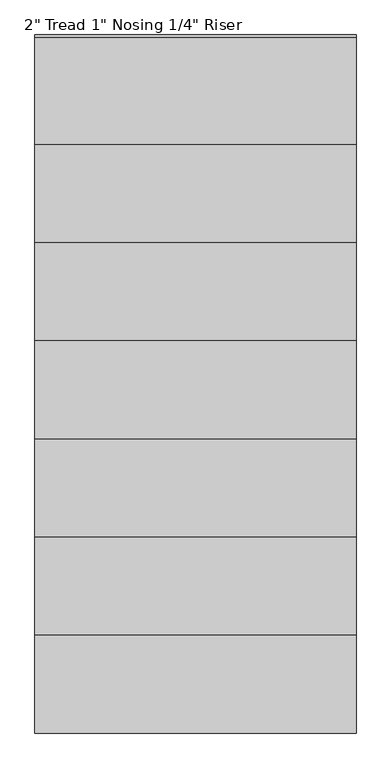
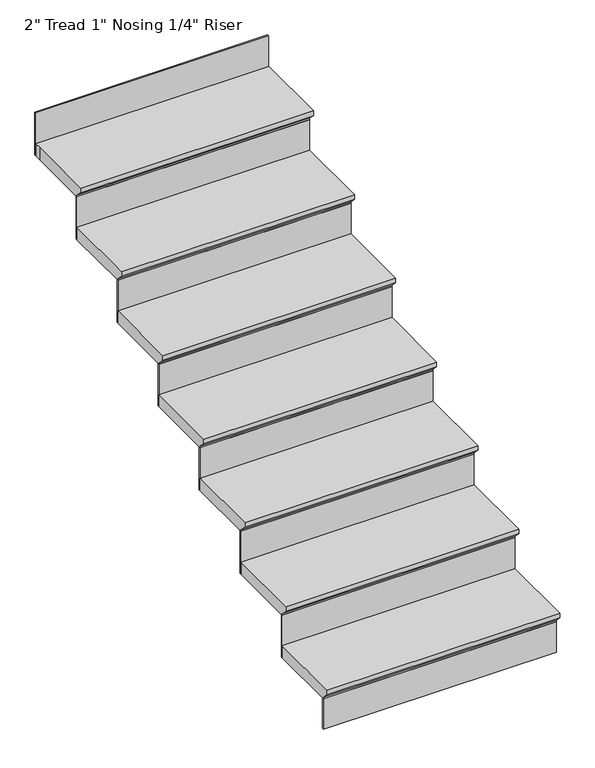
"""IFC4 building model written with IfcOpenShell, lengths in millimetres: stair flight geometry."""

from ifc_helpers import new_model, si_unit, origin, place, context, project, spatial, faceted_brep, source, transform, mapped, element, save


def stair_flight_57d74f5f(model_context):
    return source(origin(), model_context, "Body", "Brep", [
        faceted_brep([(1046.3501403, 157.6257925, 3968.75), (1046.3501403, 157.6257925, 3987.8), (131.9501403, 157.6257925, 3987.8), (131.9501403, 157.6257925, 3968.75), (1046.3501403, 183.0257925, 3943.35), (131.9501403, 183.0257925, 3943.35), (1046.3501403, 462.4257925, 3987.8), (131.9501403, 462.4257925, 3987.8), (131.9501403, 183.0257925, 3937.0), (131.9501403, 462.4257925, 3937.0), (1046.3501403, 462.4257925, 3937.0), (1046.3501403, 183.0257925, 3937.0)], [[[0, 1, 2, 3]], [[4, 0, 3, 5]], [[2, 1, 6, 7]], [[8, 9, 10, 11]], [[2, 7, 9, 8, 5, 3]], [[8, 11, 4, 5]], [[6, 1, 0, 4, 11, 10]], [[7, 6, 10, 9]]]),
        faceted_brep([(1046.3501403, 183.0257925, 3937.0), (1046.3501403, 183.0257925, 3810.0), (1046.3501403, 189.3757925, 3810.0), (1046.3501403, 189.3757925, 3937.0), (131.9501403, 183.0257925, 3937.0), (131.9501403, 189.3757925, 3937.0), (131.9501403, 189.3757925, 3810.0), (131.9501403, 183.0257925, 3810.0)], [[[0, 1, 2, 3]], [[4, 5, 6, 7]], [[1, 0, 4, 7]], [[2, 1, 7, 6]], [[3, 2, 6, 5]], [[0, 3, 5, 4]]]),
        faceted_brep([(1046.3501403, 462.4257925, 4114.8), (1046.3501403, 462.4257925, 3937.0), (1046.3501403, 468.7757925, 3937.0), (1046.3501403, 468.7757925, 4114.8), (131.9501403, 462.4257925, 4114.8), (131.9501403, 468.7757925, 4114.8), (131.9501403, 468.7757925, 3937.0), (131.9501403, 462.4257925, 3937.0)], [[[0, 1, 2, 3]], [[4, 5, 6, 7]], [[1, 0, 4, 7]], [[2, 1, 7, 6]], [[3, 2, 6, 5]], [[0, 3, 5, 4]]]),
        faceted_brep([(131.9501403, 437.0257925, 4165.6), (1046.3501403, 437.0257925, 4165.6), (1046.3501403, 741.8257925, 4165.6), (131.9501403, 741.8257925, 4165.6), (131.9501403, 462.4257925, 4114.8), (131.9501403, 741.8257925, 4114.8), (1046.3501403, 741.8257925, 4114.8), (1046.3501403, 462.4257925, 4114.8), (131.9501403, 462.4257925, 4121.15), (131.9501403, 437.0257925, 4146.55), (1046.3501403, 462.4257925, 4121.15), (1046.3501403, 437.0257925, 4146.55)], [[[0, 1, 2, 3]], [[4, 5, 6, 7]], [[0, 3, 5, 4, 8, 9]], [[4, 7, 10, 8]], [[2, 1, 11, 10, 7, 6]], [[3, 2, 6, 5]], [[11, 1, 0, 9]], [[10, 11, 9, 8]]]),
        faceted_brep([(1046.3501403, 741.8257925, 4292.6), (1046.3501403, 741.8257925, 4114.8), (1046.3501403, 748.1757925, 4114.8), (1046.3501403, 748.1757925, 4292.6), (131.9501403, 741.8257925, 4292.6), (131.9501403, 748.1757925, 4292.6), (131.9501403, 748.1757925, 4114.8), (131.9501403, 741.8257925, 4114.8)], [[[0, 1, 2, 3]], [[4, 5, 6, 7]], [[1, 0, 4, 7]], [[2, 1, 7, 6]], [[3, 2, 6, 5]], [[0, 3, 5, 4]]]),
        faceted_brep([(131.9501403, 716.4257925, 4343.4), (1046.3501403, 716.4257925, 4343.4), (1046.3501403, 1021.2257925, 4343.4), (131.9501403, 1021.2257925, 4343.4), (131.9501403, 741.8257925, 4292.6), (131.9501403, 1021.2257925, 4292.6), (1046.3501403, 1021.2257925, 4292.6), (1046.3501403, 741.8257925, 4292.6), (131.9501403, 741.8257925, 4298.95), (131.9501403, 716.4257925, 4324.35), (1046.3501403, 741.8257925, 4298.95), (1046.3501403, 716.4257925, 4324.35)], [[[0, 1, 2, 3]], [[4, 5, 6, 7]], [[0, 3, 5, 4, 8, 9]], [[4, 7, 10, 8]], [[2, 1, 11, 10, 7, 6]], [[3, 2, 6, 5]], [[11, 1, 0, 9]], [[10, 11, 9, 8]]]),
        faceted_brep([(1046.3501403, 1021.2257925, 4470.4), (1046.3501403, 1021.2257925, 4292.6), (1046.3501403, 1027.5757925, 4292.6), (1046.3501403, 1027.5757925, 4470.4), (131.9501403, 1021.2257925, 4470.4), (131.9501403, 1027.5757925, 4470.4), (131.9501403, 1027.5757925, 4292.6), (131.9501403, 1021.2257925, 4292.6)], [[[0, 1, 2, 3]], [[4, 5, 6, 7]], [[1, 0, 4, 7]], [[2, 1, 7, 6]], [[3, 2, 6, 5]], [[0, 3, 5, 4]]]),
        faceted_brep([(131.9501403, 995.8257925, 4521.2), (1046.3501403, 995.8257925, 4521.2), (1046.3501403, 1300.6257925, 4521.2), (131.9501403, 1300.6257925, 4521.2), (131.9501403, 1021.2257925, 4470.4), (131.9501403, 1300.6257925, 4470.4), (1046.3501403, 1300.6257925, 4470.4), (1046.3501403, 1021.2257925, 4470.4), (131.9501403, 1021.2257925, 4476.75), (131.9501403, 995.8257925, 4502.15), (1046.3501403, 1021.2257925, 4476.75), (1046.3501403, 995.8257925, 4502.15)], [[[0, 1, 2, 3]], [[4, 5, 6, 7]], [[0, 3, 5, 4, 8, 9]], [[4, 7, 10, 8]], [[2, 1, 11, 10, 7, 6]], [[3, 2, 6, 5]], [[11, 1, 0, 9]], [[10, 11, 9, 8]]]),
        faceted_brep([(1046.3501403, 1300.6257925, 4648.2), (1046.3501403, 1300.6257925, 4470.4), (1046.3501403, 1306.9757925, 4470.4), (1046.3501403, 1306.9757925, 4648.2), (131.9501403, 1300.6257925, 4648.2), (131.9501403, 1306.9757925, 4648.2), (131.9501403, 1306.9757925, 4470.4), (131.9501403, 1300.6257925, 4470.4)], [[[0, 1, 2, 3]], [[4, 5, 6, 7]], [[1, 0, 4, 7]], [[2, 1, 7, 6]], [[3, 2, 6, 5]], [[0, 3, 5, 4]]]),
        faceted_brep([(131.9501403, 1275.2257925, 4699.0), (1046.3501403, 1275.2257925, 4699.0), (1046.3501403, 1580.0257925, 4699.0), (131.9501403, 1580.0257925, 4699.0), (131.9501403, 1300.6257925, 4648.2), (131.9501403, 1580.0257925, 4648.2), (1046.3501403, 1580.0257925, 4648.2), (1046.3501403, 1300.6257925, 4648.2), (131.9501403, 1300.6257925, 4654.55), (131.9501403, 1275.2257925, 4679.95), (1046.3501403, 1300.6257925, 4654.55), (1046.3501403, 1275.2257925, 4679.95)], [[[0, 1, 2, 3]], [[4, 5, 6, 7]], [[0, 3, 5, 4, 8, 9]], [[4, 7, 10, 8]], [[2, 1, 11, 10, 7, 6]], [[3, 2, 6, 5]], [[11, 1, 0, 9]], [[10, 11, 9, 8]]]),
        faceted_brep([(1046.3501403, 1580.0257925, 4826.0), (1046.3501403, 1580.0257925, 4648.2), (1046.3501403, 1586.3757925, 4648.2), (1046.3501403, 1586.3757925, 4826.0), (131.9501403, 1580.0257925, 4826.0), (131.9501403, 1586.3757925, 4826.0), (131.9501403, 1586.3757925, 4648.2), (131.9501403, 1580.0257925, 4648.2)], [[[0, 1, 2, 3]], [[4, 5, 6, 7]], [[1, 0, 4, 7]], [[2, 1, 7, 6]], [[3, 2, 6, 5]], [[0, 3, 5, 4]]]),
        faceted_brep([(131.9501403, 1554.6257925, 4876.8), (1046.3501403, 1554.6257925, 4876.8), (1046.3501403, 1859.4257925, 4876.8), (131.9501403, 1859.4257925, 4876.8), (131.9501403, 1580.0257925, 4826.0), (131.9501403, 1859.4257925, 4826.0), (1046.3501403, 1859.4257925, 4826.0), (1046.3501403, 1580.0257925, 4826.0), (131.9501403, 1580.0257925, 4832.35), (131.9501403, 1554.6257925, 4857.75), (1046.3501403, 1580.0257925, 4832.35), (1046.3501403, 1554.6257925, 4857.75)], [[[0, 1, 2, 3]], [[4, 5, 6, 7]], [[0, 3, 5, 4, 8, 9]], [[4, 7, 10, 8]], [[2, 1, 11, 10, 7, 6]], [[3, 2, 6, 5]], [[11, 1, 0, 9]], [[10, 11, 9, 8]]]),
        faceted_brep([(1046.3501403, 2138.8257925, 5181.6), (1046.3501403, 2138.8257925, 5003.8), (1046.3501403, 2145.1757925, 5003.8), (1046.3501403, 2145.1757925, 5181.6), (131.9501403, 2138.8257925, 5181.6), (131.9501403, 2145.1757925, 5181.6), (131.9501403, 2145.1757925, 5003.8), (131.9501403, 2138.8257925, 5003.8)], [[[0, 1, 2, 3]], [[4, 5, 6, 7]], [[1, 0, 4, 7]], [[2, 1, 7, 6]], [[3, 2, 6, 5]], [[0, 3, 5, 4]]]),
        faceted_brep([(1046.3501403, 1859.4257925, 5003.8), (1046.3501403, 1859.4257925, 4826.0), (1046.3501403, 1865.7757925, 4826.0), (1046.3501403, 1865.7757925, 5003.8), (131.9501403, 1859.4257925, 5003.8), (131.9501403, 1865.7757925, 5003.8), (131.9501403, 1865.7757925, 4826.0), (131.9501403, 1859.4257925, 4826.0)], [[[0, 1, 2, 3]], [[4, 5, 6, 7]], [[1, 0, 4, 7]], [[2, 1, 7, 6]], [[3, 2, 6, 5]], [[0, 3, 5, 4]]]),
        faceted_brep([(131.9501403, 2138.8257925, 5054.6), (131.9501403, 2113.4257925, 5054.6), (131.9501403, 1834.0257925, 5054.6), (1046.3501403, 1834.0257925, 5054.6), (1046.3501403, 2138.8257925, 5054.6), (131.9501403, 2113.4257925, 5003.8), (131.9501403, 2138.8257925, 5003.8), (1046.3501403, 2138.8257925, 5003.8), (1046.3501403, 1859.4257925, 5003.8), (131.9501403, 1859.4257925, 5003.8), (131.9501403, 1859.4257925, 5010.15), (131.9501403, 1834.0257925, 5035.55), (1046.3501403, 1859.4257925, 5010.15), (1046.3501403, 1834.0257925, 5035.55)], [[[0, 1, 2, 3, 4]], [[5, 6, 7, 8, 9]], [[1, 0, 6, 5]], [[2, 1, 5, 9, 10, 11]], [[9, 8, 12, 10]], [[4, 3, 13, 12, 8, 7]], [[0, 4, 7, 6]], [[13, 3, 2, 11]], [[12, 13, 11, 10]]]),
    ])


if __name__ == "__main__":
    model = new_model("IFC4")
    model_context = context("Model", 3, world=origin())
    ifc_project = project(units=[si_unit("LENGTHUNIT", "METRE", prefix="MILLI")], contexts=[model_context])
    site = spatial("IfcSite", under=ifc_project)
    building = spatial("IfcBuilding", under=site)
    placement = place(None, origin())
    stair_flight_shape = stair_flight_57d74f5f(model_context)
    element("IfcStairFlight", 1, ObjectType="2\" Tread 1\" Nosing 1/4\" Riser", at=placement, inside=building, context=model_context, shape_type="MappedRepresentation", body=[
        mapped(stair_flight_shape, transform((0.0, 0.0, 0.0), x_axis=(1.0, 0.0, 0.0), y_axis=(0.0, 1.0, 0.0), z_axis=(0.0, 0.0, 1.0))),
    ])
    save(model, "model.ifc")
